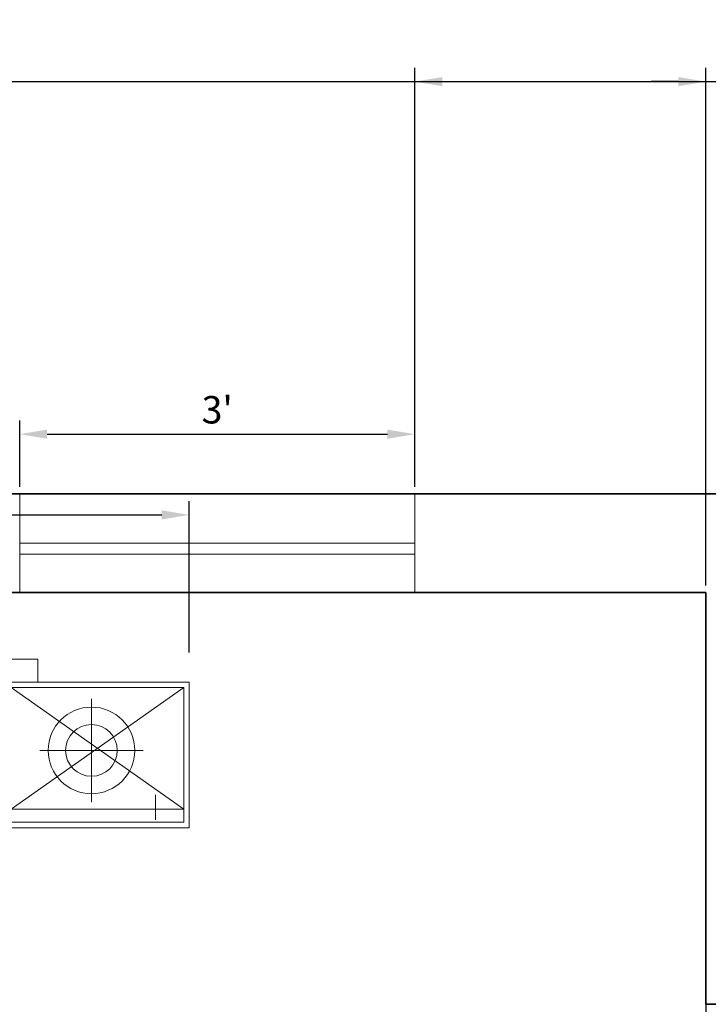
# Model space of a CAD drawing. Units: inches. Extents: x 2025 to 2528, y 1525 to 2336.
# Tile 16 of 18: x 2192 to 2255, y 2246 to 2336. Entities that reach past the tile are written whole.
import ezdxf

# ---------------------------------------------------------------- set-up
doc = ezdxf.new("R2010")
doc.units = ezdxf.units.IN
for name, color, linetype, lineweight in [('A-ANNO-DIMS', 2, 'Continuous', 18), ('A-FURN', 8, 'Continuous', 18), ('A-GLAZ', 4, 'Continuous', 18), ('A-WALL', 7, 'Continuous', 35)]:
    doc.layers.add(name, color=color, linetype=linetype, lineweight=lineweight)
doc.styles.get("Standard").update_dxf_attribs({"font": 'arial.ttf'})
doc.dimstyles.new('Copy of ISO-25', dxfattribs={"dimtxt": 2.5, "dimasz": 2.5, "dimexe": 1.25, "dimexo": 0.625, "dimtad": 1, "dimdec": 1, "dimlunit": 4, "dimtxsty": 'Standard', "dimcen": 2.5, "dimadec": 0, "dimazin": 0, "dimtfac": 1, "dimtdec": 1, "dimtmove": 0, "dimatfit": 3, "dimfxl": 1, "dimarcsym": 0})

# ---------------------------------------------------------------- blocks, each defined once
blk = doc.blocks.new('*D6')
at = {"layer": 'A-ANNO-DIMS', "color": 0, "lineweight": -2, "transparency": 16777216}
for p, q in [((2075.013, 2282.787), (2075.013, 2237.927)), ((2255.013, 2282.787), (2255.013, 2237.927)), ((2077.513, 2239.177), (2252.513, 2239.177))]:
    blk.add_line(p, q, dxfattribs=at)
at = {"layer": 'A-ANNO-DIMS', "color": 0, "transparency": 16777216}
for points in [[(2077.513, 2239.594), (2077.513, 2238.761), (2075.013, 2239.177)], [(2252.513, 2239.594), (2252.513, 2238.761), (2255.013, 2239.177)]]:
    blk.add_solid(points, dxfattribs=at)
at = {"layer": 'Defpoints', "color": 0, "transparency": 16777216}
for p in [(2075.013, 2283.412), (2255.013, 2283.412), (2255.013, 2239.177)]:
    blk.add_point(p, dxfattribs=at)
at = {"layer": 'A-ANNO-DIMS', "color": 0, "transparency": 16777216, "insert": (2165.013, 2241.079), "char_height": 2.5, "attachment_point": 5}
blk.add_mtext("15'", dxfattribs=at)
blk = doc.blocks.new('*D21')
at = {"layer": 'A-ANNO-DIMS', "color": 0, "lineweight": -2, "transparency": 16777216}
for p, q in [((2192.485, 2293.037), (2192.485, 2299.084)), ((2228.485, 2293.037), (2228.485, 2299.084)), ((2194.985, 2297.834), (2225.985, 2297.834))]:
    blk.add_line(p, q, dxfattribs=at)
at = {"layer": 'A-ANNO-DIMS', "color": 0, "transparency": 16777216}
for points in [[(2194.985, 2298.25), (2194.985, 2297.417), (2192.485, 2297.834)], [(2225.985, 2298.25), (2225.985, 2297.417), (2228.485, 2297.834)]]:
    blk.add_solid(points, dxfattribs=at)
at = {"layer": 'Defpoints', "color": 0, "transparency": 16777216}
for p in [(2228.485, 2297.834), (2192.485, 2292.412), (2228.485, 2292.412)]:
    blk.add_point(p, dxfattribs=at)
at = {"layer": 'A-ANNO-DIMS', "color": 0, "transparency": 16777216, "insert": (2210.485, 2299.736), "char_height": 2.5, "attachment_point": 5}
blk.add_mtext("3'", dxfattribs=at)
blk = doc.blocks.new('A$C029D5C69')
for p, q in [((2.2315, 2.0693), (0.4164, 2.0693)), ((2.2315, 2.0066), (2.2315, 2.0693)), ((0.4164, 2.0066), (2.2315, 2.0066)), ((2.6479, 2.0066), (2.1429, 2.0066)), ((2.6479, 1.606), (2.6479, 2.0066)), ((2.6328, 1.9915), (2.158, 1.9915)), ((2.6328, 1.6211), (2.6328, 1.9915)), ((2.379, 1.9609), (2.379, 1.6764)), ((2.2367, 1.8186), (2.5212, 1.8186)), ((2.5551, 1.6275), (2.5551, 1.696)), ((2.1429, 1.606), (2.6479, 1.606)), ((2.158, 1.6211), (2.6328, 1.6211))]:
    blk.add_line(p, q)
at = {"ltscale": 0.005}
for p, q in [((2.6328, 1.6568), (2.158, 1.9915)), ((2.158, 1.6568), (2.6328, 1.9915)), ((2.6328, 1.6568), (2.158, 1.6568))]:
    blk.add_line(p, q, dxfattribs=at)
for radius in [0.1191, 0.0711]:
    blk.add_circle((2.379, 1.8186), radius)
blk = doc.blocks.new('WIN-36-EXT')
for p, q in [((0, 0), (0, 9)), ((0, 9), (36, 9)), ((36, 9), (36, 0)), ((0, 4.5), (36, 4.5)), ((0, 3.5), (36, 3.5))]:
    blk.add_line(p, q)
blk = doc.blocks.new('*D56')
at = {"layer": 'A-ANNO-DIMS', "color": 0, "lineweight": -2, "transparency": 16777216}
for p, q in [((2120.208, 2277.944), (2120.208, 2291.728)), ((2207.933, 2277.944), (2207.933, 2291.728)), ((2122.708, 2290.478), (2205.433, 2290.478))]:
    blk.add_line(p, q, dxfattribs=at)
at = {"layer": 'A-ANNO-DIMS', "color": 0, "transparency": 16777216}
for points in [[(2122.708, 2290.895), (2122.708, 2290.061), (2120.208, 2290.478)], [(2205.433, 2290.895), (2205.433, 2290.061), (2207.933, 2290.478)]]:
    blk.add_solid(points, dxfattribs=at)
at = {"layer": 'Defpoints', "color": 0, "transparency": 16777216}
for p in [(2207.933, 2290.478), (2120.208, 2277.319), (2207.933, 2277.319)]:
    blk.add_point(p, dxfattribs=at)
at = {"layer": 'A-ANNO-DIMS', "color": 0, "transparency": 16777216, "insert": (2164.07, 2292.403), "char_height": 2.5, "attachment_point": 5}
blk.add_mtext('BED & NIGHTSTANDS 7\'-3 1/2" TYP.', dxfattribs=at)
blk = doc.blocks.new('*D62')
at = {"layer": 'A-ANNO-DIMS', "color": 0, "lineweight": -2, "transparency": 16777216}
for p, q in [((2228.485, 2293.037), (2228.485, 2331.212)), ((2318.013, 2293.037), (2318.013, 2331.212)), ((2230.985, 2329.962), (2315.513, 2329.962))]:
    blk.add_line(p, q, dxfattribs=at)
at = {"layer": 'A-ANNO-DIMS', "color": 0, "transparency": 16777216}
for points in [[(2230.985, 2330.379), (2230.985, 2329.546), (2228.485, 2329.962)], [(2315.513, 2330.379), (2315.513, 2329.546), (2318.013, 2329.962)]]:
    blk.add_solid(points, dxfattribs=at)
at = {"layer": 'Defpoints', "color": 0, "transparency": 16777216}
for p in [(2318.013, 2329.962), (2228.485, 2292.412), (2318.013, 2292.412)]:
    blk.add_point(p, dxfattribs=at)
at = {"layer": 'A-ANNO-DIMS', "color": 0, "transparency": 16777216, "insert": (2273.249, 2331.88), "char_height": 2.5, "attachment_point": 5}
blk.add_mtext('7\'-5 1/2"', dxfattribs=at)
blk = doc.blocks.new('*D74')
at = {"layer": 'A-ANNO-DIMS', "color": 0, "lineweight": -2, "transparency": 16777216}
for p, q in [((2255.013, 2284.037), (2255.013, 2331.212)), ((2261.013, 2284.037), (2261.013, 2331.212)), ((2252.513, 2329.962), (2250.013, 2329.962)), ((2255.013, 2329.962), (2261.013, 2329.962)), ((2263.513, 2329.962), (2273.909, 2329.962))]:
    blk.add_line(p, q, dxfattribs=at)
at = {"layer": 'A-ANNO-DIMS', "color": 0, "transparency": 16777216}
for points in [[(2252.513, 2330.379), (2252.513, 2329.546), (2255.013, 2329.962)], [(2263.513, 2330.379), (2263.513, 2329.546), (2261.013, 2329.962)]]:
    blk.add_solid(points, dxfattribs=at)
at = {"layer": 'Defpoints', "color": 0, "transparency": 16777216}
for p in [(2261.013, 2329.962), (2255.013, 2283.412), (2261.013, 2283.412)]:
    blk.add_point(p, dxfattribs=at)
at = {"layer": 'A-ANNO-DIMS', "color": 0, "transparency": 16777216, "insert": (2269.961, 2331.864), "char_height": 2.5, "attachment_point": 5}
blk.add_mtext('0\'-6"', dxfattribs=at)
blk = doc.blocks.new('*D79')
at = {"layer": 'A-ANNO-DIMS', "color": 0, "lineweight": -2, "transparency": 16777216}
for p, q in [((2066.013, 2293.037), (2066.013, 2331.212)), ((2489.013, 2293.037), (2489.013, 2331.212)), ((2068.513, 2329.962), (2486.513, 2329.962))]:
    blk.add_line(p, q, dxfattribs=at)
at = {"layer": 'A-ANNO-DIMS', "color": 0, "transparency": 16777216}
for points in [[(2068.513, 2330.379), (2068.513, 2329.546), (2066.013, 2329.962)], [(2486.513, 2330.379), (2486.513, 2329.546), (2489.013, 2329.962)]]:
    blk.add_solid(points, dxfattribs=at)
at = {"layer": 'Defpoints', "color": 0, "transparency": 16777216}
for p in [(2489.013, 2329.962), (2066.013, 2292.412), (2489.013, 2292.412)]:
    blk.add_point(p, dxfattribs=at)
at = {"layer": 'A-ANNO-DIMS', "color": 0, "transparency": 16777216, "insert": (2277.513, 2331.865), "char_height": 2.5, "attachment_point": 5}
blk.add_mtext('35\'-3"', dxfattribs=at)
blk = doc.blocks.new('*D80')
at = {"layer": 'A-ANNO-DIMS', "color": 0, "lineweight": -2, "transparency": 16777216}
for p, q in [((2065.388, 2292.412), (2027.213, 2292.412)), ((2028.463, 1566.912), (2028.463, 2289.912)), ((2285.388, 1564.412), (2027.213, 1564.412))]:
    blk.add_line(p, q, dxfattribs=at)
at = {"layer": 'A-ANNO-DIMS', "color": 0, "transparency": 16777216}
for points in [[(2028.046, 2289.912), (2028.88, 2289.912), (2028.463, 2292.412)], [(2028.046, 1566.912), (2028.88, 1566.912), (2028.463, 1564.412)]]:
    blk.add_solid(points, dxfattribs=at)
at = {"layer": 'Defpoints', "color": 0, "transparency": 16777216}
for p in [(2028.463, 2292.412), (2066.013, 2292.412), (2286.013, 1564.412)]:
    blk.add_point(p, dxfattribs=at)
at = {"layer": 'A-ANNO-DIMS', "color": 0, "transparency": 16777216, "insert": (2026.561, 1928.412), "char_height": 2.5, "attachment_point": 5, "rotation": 90}
blk.add_mtext('60\'-8"', dxfattribs=at)

msp = doc.modelspace()

# ---------------------------------------------------------------- linework, layer by layer
at = {"layer": 'A-WALL'}
for p, q in [((2066.013, 2292.412), (2246.013, 2292.412)), ((2246.013, 2292.412), (2252.013, 2292.412)), ((2252.013, 2292.412), (2312.013, 2292.412)), ((2075.013, 2283.412), (2246.013, 2283.412)), ((2075.013, 2283.412), (2255.013, 2283.412)), ((2255.013, 2283.412), (2228.485, 2283.412)), ((2246.013, 2283.412), (2252.013, 2283.412)), ((2252.013, 2283.412), (2255.013, 2283.412)), ((2255.013, 2283.412), (2255.013, 2245.877)), ((2255.013, 2283.412), (2255.013, 2245.877)), ((2255.013, 2245.877), (2261.013, 2245.877))]:
    msp.add_line(p, q, dxfattribs=at)

# ---------------------------------------------------------------- block references
at = {"layer": 'A-FURN', "xscale": 33.13032201413296, "yscale": 33.13032201413296, "zscale": 33.13032201413296}
msp.add_blockref('A$C029D5C69', (2120.208, 2208.764), dxfattribs=at)
at = {"layer": 'A-GLAZ'}
msp.add_blockref('WIN-36-EXT', (2192.485, 2283.412), dxfattribs=at)

# ---------------------------------------------------------------- dimensions: what is measured, and where the dimension line sits
at = {"layer": 'A-ANNO-DIMS'}
for base, p1, p2, override, picture, middle in [((2318.013, 2329.962), (2228.485, 2292.412), (2318.013, 2292.412), {"dimdec": 1, "dimlfac": 1, "dimrnd": 0, "dimzin": 1, "dimdsep": 46, "dimlunit": 4, "dimfrac": 2}, '*D62', (2273.249, 2331.88)), ((2489.013, 2329.962), (2066.013, 2292.412), (2489.013, 2292.412), {"dimdec": 1, "dimlfac": 1, "dimrnd": 0, "dimzin": 1, "dimdsep": 46, "dimlunit": 4, "dimfrac": 2}, '*D79', (2277.513, 2331.865)), ((2261.013, 2329.962), (2255.013, 2283.412), (2261.013, 2283.412), {"dimdec": 1, "dimlfac": 1, "dimrnd": 0, "dimzin": 1, "dimdsep": 46, "dimlunit": 4, "dimfrac": 2}, '*D74', (2269.961, 2331.864)), ((2228.485, 2297.834), (2192.485, 2292.412), (2228.485, 2292.412), {"dimclrd": 0, "dimclre": 0, "dimclrt": 0}, '*D21', (2210.485, 2299.736)), ((2255.013, 2239.177), (2075.013, 2283.412), (2255.013, 2283.412), {"dimclrd": 0, "dimclre": 0, "dimclrt": 0}, '*D6', (2165.013, 2241.079))]:
    dim = msp.add_linear_dim(base=base, p1=p1, p2=p2, dimstyle='Copy of ISO-25', override=override, dxfattribs=at)
    dim.commit()
    dim.dimension.update_dxf_attribs({"geometry": picture, "text_midpoint": middle})
dim = msp.add_linear_dim(base=(2207.933, 2290.478), p1=(2120.208, 2277.319), p2=(2207.933, 2277.319), text='BED & NIGHTSTANDS <> TYP.', dimstyle='Copy of ISO-25', override={"dimdec": 1, "dimlfac": 1, "dimrnd": 0, "dimzin": 1, "dimdsep": 46, "dimlunit": 4, "dimfrac": 2}, dxfattribs=at)
dim.commit()
dim.dimension.update_dxf_attribs({"geometry": '*D56', "text_midpoint": (2164.07, 2292.403)})
dim = msp.add_linear_dim(base=(2028.463, 2292.412), p1=(2286.013, 1564.412), p2=(2066.013, 2292.412), angle=90, dimstyle='Copy of ISO-25', override={"dimdec": 1, "dimlfac": 1, "dimrnd": 0, "dimzin": 1, "dimdsep": 46, "dimlunit": 4, "dimfrac": 2}, dxfattribs=at)
dim.commit()
dim.dimension.update_dxf_attribs({"geometry": '*D80', "text_midpoint": (2026.561, 1928.412)})

doc.saveas('drawing.dxf')
